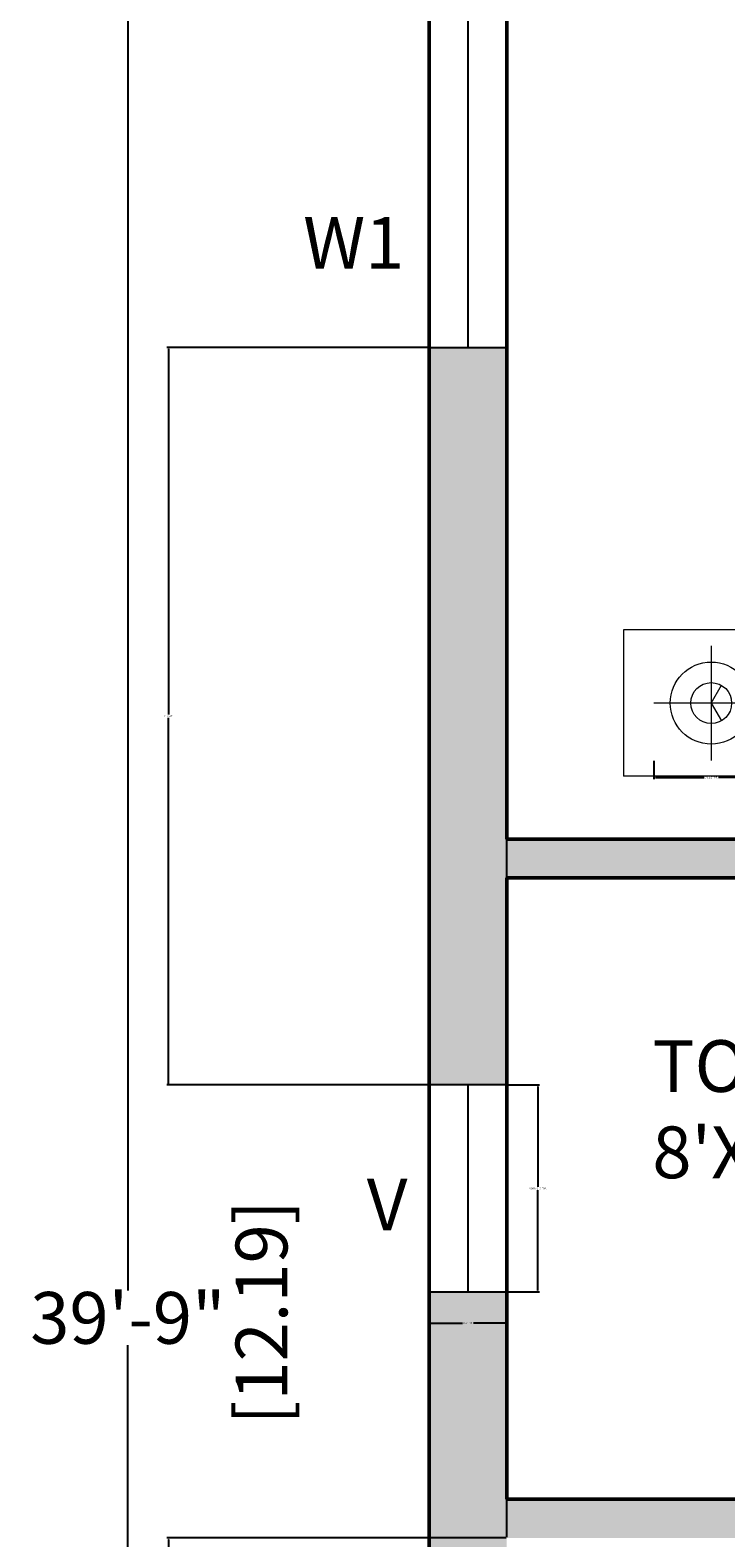
# Model space of a CAD drawing. Units: inches. Extents: x -15 to 420, y -514 to 86.
# Tile 4 of 8: x -15 to 65, y -251 to -76. Entities that reach past the tile are written whole.
import ezdxf

# ---------------------------------------------------------------- set-up
doc = ezdxf.new("R2010")
doc.units = ezdxf.units.IN
doc.header["$MEASUREMENT"] = 0
for name, color, linetype, lineweight in [('A-ANNO-DIMS', 2, 'Continuous', 18), ('A-ANNO-TEXT', 7, 'Continuous', 18), ('A-AREA-IDEN', 7, 'Continuous', 25), ('A-FURN', 8, 'Continuous', 18), ('A-GLAZ', 41, 'Continuous', 25), ('A-WALL', 7, 'Continuous', 50), ('A-WALL-PATT', 8, 'Continuous', 13)]:
    doc.layers.add(name, color=color, linetype=linetype, lineweight=lineweight)
doc.styles.get("Standard").update_dxf_attribs({"font": 'arial.ttf'})
doc.dimstyles.get("Standard").update_dxf_attribs({"dimtxt": 0.18, "dimasz": 0.18, "dimexe": 0.18, "dimexo": 0.0625, "dimgap": 0.09, "dimtad": 0, "dimtih": 1, "dimtoh": 1, "dimdec": 0, "dimzin": 0, "dimdsep": 46, "dimlunit": 3, "dimtxsty": 'Standard', "dimcen": 0.09, "dimadec": 0, "dimazin": 0, "dimtfac": 1, "dimtdec": 0, "dimtofl": 0, "dimtmove": 0, "dimatfit": 3, "dimfxl": 1, "dimtolj": 1, "dimtzin": 0, "dimarcsym": 0})

# ---------------------------------------------------------------- blocks, each defined once
blk = doc.blocks.new('*D2')
at = {"layer": 'A-ANNO-DIMS', "color": 0, "lineweight": -2, "transparency": 16777216}
for p, q in [((30.86, 13.12), (-4.15, 13.12)), ((-3.97, 12.94), (-3.97, -222.22)), ((-3.97, -463.7), (-3.97, -228.53)), ((30.86, -463.88), (-4.15, -463.88))]:
    blk.add_line(p, q, dxfattribs=at)
at = {"layer": 'A-ANNO-DIMS', "color": 0, "transparency": 16777216}
for points in [[(-4, 12.94), (-3.94, 12.94), (-3.97, 13.12)], [(-4, -463.7), (-3.94, -463.7), (-3.97, -463.88)]]:
    blk.add_solid(points, dxfattribs=at)
at = {"layer": 'Defpoints', "color": 0, "transparency": 16777216}
for p in [(30.92, 13.12), (-3.97, -463.88), (30.92, -463.88)]:
    blk.add_point(p, dxfattribs=at)
at = {"layer": 'A-ANNO-DIMS', "color": 0, "transparency": 16777216, "insert": (-3.97, -225.38), "char_height": 6, "attachment_point": 5}
blk.add_mtext('\\A1;39\'-9"', dxfattribs=at)
blk = doc.blocks.new('WIN-W1-60IN')
for p, q in [((0, 60), (0, 0)), ((4.5, 60), (4.5, 0)), ((9, 0), (9, 60))]:
    blk.add_line(p, q)
blk = doc.blocks.new('VENT-V-24IN')
for p, q in [((0, 24), (0, 0)), ((4.5, 24), (4.5, 0)), ((9, 0), (9, 24))]:
    blk.add_line(p, q)
blk = doc.blocks.new('BEDSIDE-LAMP-9-5IN')
for p, q in [((6.64, 13.29), (6.64, 0)), ((13.29, 6.64), (0, 6.64))]:
    blk.add_line(p, q)
for points in [[(6.64, 6.64), (7.83, 8.7)], [(6.64, 6.64), (7.83, 4.59)]]:
    blk.add_lwpolyline(points)
for radius in [4.75, 2.37]:
    blk.add_circle((6.64, 6.64), radius)
blk = doc.blocks.new('*D19')
at = {"layer": 'A-ANNO-DIMS', "color": 0, "lineweight": -2, "transparency": 16777216}
for p, q in [((39.99, -198.38), (43.7, -198.38)), ((43.52, -198.56), (43.52, -210.2)), ((43.52, -222.2), (43.52, -210.56)), ((39.99, -222.38), (43.7, -222.38))]:
    blk.add_line(p, q, dxfattribs=at)
at = {"layer": 'A-ANNO-DIMS', "color": 0, "transparency": 16777216}
for points in [[(43.49, -198.56), (43.55, -198.56), (43.52, -198.38)], [(43.49, -222.2), (43.55, -222.2), (43.52, -222.38)]]:
    blk.add_solid(points, dxfattribs=at)
at = {"layer": 'Defpoints', "color": 0, "transparency": 16777216}
for p in [(39.92, -198.38), (43.52, -198.38), (39.92, -222.38)]:
    blk.add_point(p, dxfattribs=at)
at = {"layer": 'A-ANNO-DIMS', "color": 0, "transparency": 16777216, "insert": (43.52, -210.38), "char_height": 0.18, "attachment_point": 5}
blk.add_mtext('\\A1;VENT V 2\'-0" TYP.', dxfattribs=at)
blk = doc.blocks.new('*D20')
at = {"layer": 'A-ANNO-DIMS', "color": 0, "lineweight": -2, "transparency": 16777216}
for p, q in [((30.92, -222.44), (30.92, -226.16)), ((39.92, -222.44), (39.92, -226.16)), ((31.1, -225.98), (34.79, -225.98)), ((39.74, -225.98), (36.06, -225.98))]:
    blk.add_line(p, q, dxfattribs=at)
at = {"layer": 'A-ANNO-DIMS', "color": 0, "transparency": 16777216}
for points in [[(31.1, -225.95), (31.1, -226.01), (30.92, -225.98)], [(39.74, -225.95), (39.74, -226.01), (39.92, -225.98)]]:
    blk.add_solid(points, dxfattribs=at)
at = {"layer": 'Defpoints', "color": 0, "transparency": 16777216}
for p in [(30.92, -222.38), (39.92, -222.38), (39.92, -225.98)]:
    blk.add_point(p, dxfattribs=at)
at = {"layer": 'A-ANNO-DIMS', "color": 0, "transparency": 16777216, "insert": (35.42, -225.98), "char_height": 0.18, "attachment_point": 5}
blk.add_mtext('\\A1;0\'-9" TYP.', dxfattribs=at)
blk = doc.blocks.new('*D36')
at = {"layer": 'A-ANNO-DIMS', "color": 0, "lineweight": -2, "transparency": 16777216}
for p, q in [((56.95, -160.81), (56.95, -162.92)), ((70.24, -160.81), (70.24, -162.92)), ((57.13, -162.74), (62.76, -162.74)), ((70.06, -162.74), (64.44, -162.74))]:
    blk.add_line(p, q, dxfattribs=at)
at = {"layer": 'A-ANNO-DIMS', "color": 0, "transparency": 16777216}
for points in [[(57.13, -162.71), (57.13, -162.77), (56.95, -162.74)], [(70.06, -162.71), (70.06, -162.77), (70.24, -162.74)]]:
    blk.add_solid(points, dxfattribs=at)
at = {"layer": 'Defpoints', "color": 0, "transparency": 16777216}
for p in [(56.95, -160.75), (70.24, -160.75), (70.24, -162.74)]:
    blk.add_point(p, dxfattribs=at)
at = {"layer": 'A-ANNO-DIMS', "color": 0, "transparency": 16777216, "insert": (63.6, -162.74), "char_height": 0.18, "attachment_point": 5}
blk.add_mtext('\\A1;1\'-1 1/2" TYP.', dxfattribs=at)
blk = doc.blocks.new('*D48')
at = {"layer": 'A-ANNO-DIMS', "color": 0, "lineweight": -2, "transparency": 16777216}
for p, q in [((39.92, -250.82), (39.92, 43.5)), ((40.1, 43.32), (56.61, 43.32)), ((74.33, 43.32), (57.83, 43.32)), ((74.51, -250.82), (74.51, 43.5))]:
    blk.add_line(p, q, dxfattribs=at)
at = {"layer": 'A-ANNO-DIMS', "color": 0, "transparency": 16777216}
for points in [[(40.1, 43.35), (40.1, 43.29), (39.92, 43.32)], [(74.33, 43.35), (74.33, 43.29), (74.51, 43.32)]]:
    blk.add_solid(points, dxfattribs=at)
at = {"layer": 'Defpoints', "color": 0, "transparency": 16777216}
for p in [(74.51, 43.32), (39.92, -250.88), (74.51, -250.88)]:
    blk.add_point(p, dxfattribs=at)
at = {"layer": 'A-ANNO-DIMS', "color": 0, "transparency": 16777216, "insert": (57.22, 43.32), "char_height": 0.18, "attachment_point": 5}
blk.add_mtext('\\A1;2\'-10 1/2"', dxfattribs=at)
blk = doc.blocks.new('*D50')
at = {"layer": 'A-ANNO-DIMS', "color": 0, "lineweight": -2, "transparency": 16777216}
for p, q in [((39.86, -250.88), (0.54, -250.88)), ((0.72, -251.06), (0.72, -290.45)), ((0.72, -330.2), (0.72, -290.81)), ((39.86, -330.38), (0.54, -330.38))]:
    blk.add_line(p, q, dxfattribs=at)
at = {"layer": 'A-ANNO-DIMS', "color": 0, "transparency": 16777216}
for points in [[(0.69, -251.06), (0.75, -251.06), (0.72, -250.88)], [(0.69, -330.2), (0.75, -330.2), (0.72, -330.38)]]:
    blk.add_solid(points, dxfattribs=at)
at = {"layer": 'Defpoints', "color": 0, "transparency": 16777216}
for p in [(39.92, -250.88), (0.72, -330.38), (39.92, -330.38)]:
    blk.add_point(p, dxfattribs=at)
at = {"layer": 'A-ANNO-DIMS', "color": 0, "transparency": 16777216, "insert": (0.72, -290.63), "char_height": 0.18, "attachment_point": 5}
blk.add_mtext('\\A1;6\'-7 1/2"', dxfattribs=at)
blk = doc.blocks.new('*D63')
at = {"layer": 'A-ANNO-DIMS', "color": 0, "lineweight": -2, "transparency": 16777216}
for p, q in [((30.86, -112.88), (0.54, -112.88)), ((0.72, -113.06), (0.72, -155.45)), ((0.72, -198.2), (0.72, -155.81)), ((30.86, -198.38), (0.54, -198.38))]:
    blk.add_line(p, q, dxfattribs=at)
at = {"layer": 'A-ANNO-DIMS', "color": 0, "transparency": 16777216}
for points in [[(0.69, -113.06), (0.75, -113.06), (0.72, -112.88)], [(0.69, -198.2), (0.75, -198.2), (0.72, -198.38)]]:
    blk.add_solid(points, dxfattribs=at)
at = {"layer": 'Defpoints', "color": 0, "transparency": 16777216}
for p in [(0.72, -112.88), (30.92, -112.88), (30.92, -198.38)]:
    blk.add_point(p, dxfattribs=at)
at = {"layer": 'A-ANNO-DIMS', "color": 0, "transparency": 16777216, "insert": (0.72, -155.63), "char_height": 0.18, "attachment_point": 5}
blk.add_mtext('\\A1;7\'-1 1/2"', dxfattribs=at)

msp = doc.modelspace()

# ---------------------------------------------------------------- hatches: boundary and pattern name
at = {"layer": 'A-WALL-PATT'}
h = msp.add_hatch(color=256, dxfattribs=at)
h.dxf.hatch_style = 1
h.paths.add_polyline_path([(266.67, -454.88), (240.92, -454.88), (240.92, -330.38), (236.42, -330.38), (236.42, -454.88), (218.42, -454.88), (218.42, -463.88), (266.67, -463.88)])
h.paths.add_polyline_path([(158.42, -454.88), (140.42, -454.88), (140.42, -394.88), (135.92, -394.88), (135.92, -454.88), (39.92, -454.88), (39.92, -412.88), (30.92, -412.88), (30.92, -463.88), (158.42, -463.88)])
h.paths.add_polyline_path([(39.92, -334.88), (135.92, -334.88), (135.92, -357.15), (140.42, -357.15), (140.42, -334.88), (173.95, -334.88), (173.95, -330.38), (39.92, -330.38), (39.92, -250.88), (155.51, -250.88), (155.51, -246.38), (140.42, -246.38), (140.42, -205.38), (138.17, -205.38), (135.92, -205.38), (135.92, -246.38), (39.92, -246.38), (39.92, -222.38), (30.92, -222.38), (30.92, -376.88), (39.92, -376.88)])
h.paths.add_polyline_path([(389.42, -382.88), (380.42, -382.88), (380.42, -454.88), (380.42, -463.88), (389.42, -463.88)])
h.paths.add_polyline_path([(352.42, -459.38), (352.42, -454.88), (326.67, -454.88), (326.67, -463.88), (352.42, -463.88)])
h.paths.add_polyline_path([(176.92, -169.88), (39.92, -169.88), (39.92, -112.88), (30.92, -112.88), (30.92, -198.38), (39.92, -198.38), (39.92, -174.38), (135.92, -174.38), (135.92, -177.38), (140.42, -177.38), (140.42, -174.38), (176.92, -174.38), (176.92, -172.13)])
h.paths.add_polyline_path([(39.92, 4.12), (93.92, 4.12), (93.92, 13.12), (30.92, 13.12), (30.92, -52.88), (39.92, -52.88)])
h.paths.add_polyline_path([(266.42, 13.12), (153.92, 13.12), (153.92, 4.12), (207.92, 4.12), (207.92, -169.88), (204.92, -169.88), (204.92, -174.38), (215.42, -174.38), (215.42, -169.88), (212.42, -169.88), (212.42, 4.12), (266.42, 4.12)])
h.paths.add_polyline_path([(389.42, 13.12), (326.42, 13.12), (326.42, 4.12), (380.42, 4.12), (380.42, -52.88), (389.42, -52.88)])
h.paths.add_polyline_path([(389.42, -112.88), (380.42, -112.88), (380.42, -169.88), (377.42, -169.88), (377.42, -174.38), (380.42, -174.38), (380.42, -198.38), (389.42, -198.38)])
h.paths.add_polyline_path([(349.42, -172.13), (349.42, -169.88), (243.42, -169.88), (243.42, -172.13), (243.42, -174.38), (279.92, -174.38), (279.92, -250.88), (380.42, -250.88), (380.42, -322.88), (389.42, -322.88), (389.42, -222.38), (380.42, -222.38), (380.42, -246.38), (284.42, -246.38), (284.42, -174.38), (349.42, -174.38)])

# ---------------------------------------------------------------- linework, layer by layer
at = {"layer": 'A-FURN'}
msp.add_line((155.11, -162.58), (53.43, -162.58), dxfattribs=at)
msp.add_lwpolyline([(73.77, -162.58), (73.77, -145.63), (53.43, -145.63), (53.43, -162.58)], dxfattribs=at)
at = {"layer": 'A-GLAZ'}
for p, q in [((30.92, -112.88), (39.92, -112.88)), ((39.92, -198.38), (30.92, -198.38)), ((30.92, -222.38), (39.92, -222.38))]:
    msp.add_line(p, q, dxfattribs=at)
at = {"layer": 'A-WALL'}
for p, q in [((30.92, 13.12), (30.92, -463.88)), ((39.92, 4.12), (39.92, -169.88)), ((39.92, -169.88), (176.92, -169.88)), ((39.92, -174.38), (135.92, -174.38)), ((39.92, -174.38), (39.92, -246.38)), ((39.92, -246.38), (135.92, -246.38))]:
    msp.add_line(p, q, dxfattribs=at)

# ---------------------------------------------------------------- block references
at = {"layer": 'A-FURN'}
msp.add_blockref('BEDSIDE-LAMP-9-5IN', (56.95, -160.75), dxfattribs=at)
at = {"layer": 'A-GLAZ'}
for name, p in [('WIN-W1-60IN', (30.92, -112.88)), ('VENT-V-24IN', (30.92, -222.38))]:
    msp.add_blockref(name, p, dxfattribs=at)

# ---------------------------------------------------------------- texts
at = {"layer": 'A-ANNO-DIMS', "insert": (8.51, -237.74), "char_height": 6, "attachment_point": 1, "rotation": 90}
msp.add_mtext_dynamic_manual_height_columns('[12.19]', width=33.4799, gutter_width=1, heights=[0], dxfattribs=at)
at = {"layer": 'A-ANNO-TEXT', "char_height": 6, "attachment_point": 1}
for s, insert in [('W1', (16.33, -97.77)), ('V', (23.7, -209.25))]:
    msp.add_mtext(s, dxfattribs=dict(at, insert=insert))
at = {"layer": 'A-AREA-IDEN', "insert": (56.77, -193.19), "char_height": 6, "attachment_point": 1}
msp.add_mtext("TOILET\\P8'X6'", dxfattribs=at)

# ---------------------------------------------------------------- dimensions: what is measured, and where the dimension line sits
at = {"layer": 'A-ANNO-DIMS'}
dim = msp.add_linear_dim(base=(74.51, 43.32), p1=(39.92, -250.88), p2=(74.51, -250.88), dimstyle='Standard', override={"dimdec": 1, "dimlfac": 1, "dimrnd": 0, "dimzin": 1, "dimdsep": 46, "dimlunit": 4, "dimfrac": 2}, dxfattribs=at)
dim.commit()
dim.dimension.update_dxf_attribs({"geometry": '*D48', "text_midpoint": (57.22, 43.32)})
for base, p1, p2, override, picture, middle in [((-3.97, -463.88), (30.92, 13.12), (30.92, -463.88), {"dimtxt": 6, "dimclrd": 0, "dimclre": 0, "dimclrt": 0}, '*D2', (-3.97, -225.38)), ((0.72, -112.88), (30.92, -198.38), (30.92, -112.88), {"dimdec": 1, "dimlfac": 1, "dimrnd": 0, "dimzin": 1, "dimdsep": 46, "dimlunit": 4, "dimfrac": 2}, '*D63', (0.72, -155.63)), ((0.72, -330.38), (39.92, -250.88), (39.92, -330.38), {"dimdec": 1, "dimlfac": 1, "dimrnd": 0, "dimzin": 1, "dimdsep": 46, "dimlunit": 4, "dimfrac": 2}, '*D50', (0.72, -290.63))]:
    dim = msp.add_linear_dim(base=base, p1=p1, p2=p2, angle=90, dimstyle='Standard', override=override, dxfattribs=at)
    dim.commit()
    dim.dimension.update_dxf_attribs({"geometry": picture, "text_midpoint": middle})
for base, p1, p2, picture, middle in [((70.24, -162.74), (56.95, -160.75), (70.24, -160.75), '*D36', (63.6, -162.74)), ((39.92, -225.98), (30.92, -222.38), (39.92, -222.38), '*D20', (35.42, -225.98))]:
    dim = msp.add_linear_dim(base=base, p1=p1, p2=p2, text='<> TYP.', dimstyle='Standard', override={"dimdec": 1, "dimlfac": 1, "dimrnd": 0, "dimzin": 1, "dimdsep": 46, "dimlunit": 4, "dimfrac": 2}, dxfattribs=at)
    dim.commit()
    dim.dimension.update_dxf_attribs({"geometry": picture, "text_midpoint": middle})
dim = msp.add_linear_dim(base=(43.52, -198.38), p1=(39.92, -222.38), p2=(39.92, -198.38), angle=90, text='VENT V <> TYP.', dimstyle='Standard', override={"dimdec": 1, "dimlfac": 1, "dimrnd": 0, "dimzin": 1, "dimdsep": 46, "dimlunit": 4, "dimfrac": 2}, dxfattribs=at)
dim.commit()
dim.dimension.update_dxf_attribs({"geometry": '*D19', "text_midpoint": (43.52, -210.38)})

doc.saveas('drawing.dxf')
